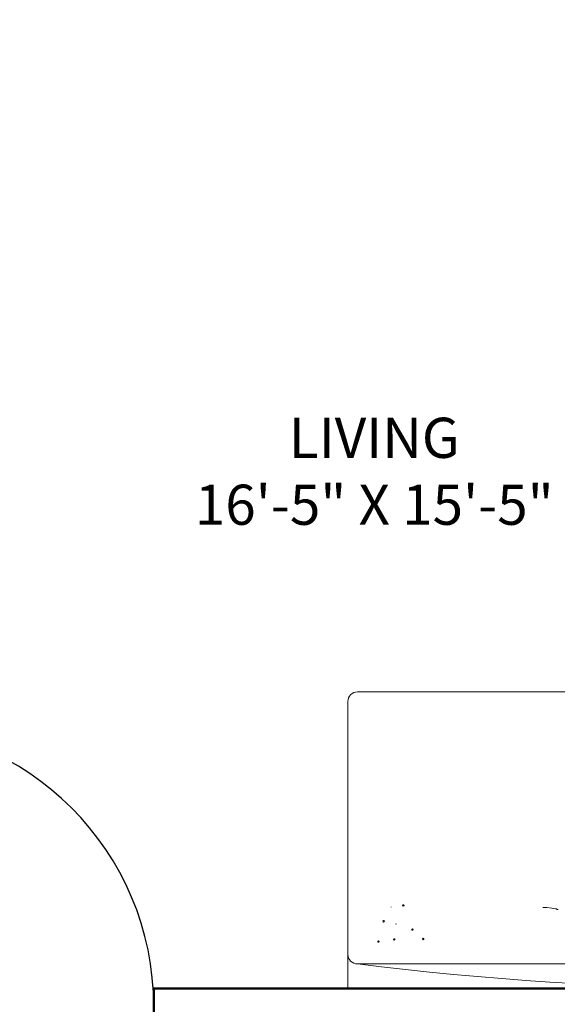
# Model space of a CAD drawing. Units: inches. Extents: x -466983 to 1020, y 324 to 318697.
# Tile 19 of 97: x 641 to 721, y 511 to 658. Entities that reach past the tile are written whole.
import ezdxf

# ---------------------------------------------------------------- set-up
doc = ezdxf.new("R2010")
doc.units = ezdxf.units.IN
doc.header["$MEASUREMENT"] = 0
for name, color, linetype, lineweight in [('A-ANNO-DIMS', 2, 'Continuous', 18), ('A-AREA-IDEN', 7, 'Continuous', 25), ('A-DOOR', 3, 'Continuous', 25), ('A-FLOR-PATT', 252, 'Continuous', 13), ('A-FURN', 8, 'Continuous', 18), ('A-WALL', 7, 'Continuous', 50)]:
    doc.layers.add(name, color=color, linetype=linetype, lineweight=lineweight)
doc.styles.get("Standard").update_dxf_attribs({"font": 'arial.ttf'})
doc.dimstyles.get("Standard").update_dxf_attribs({"dimtxt": 6, "dimasz": 4, "dimexe": 3, "dimexo": 3, "dimgap": 0.09, "dimtad": 0, "dimtih": 1, "dimtoh": 1, "dimdec": 1, "dimzin": 0, "dimdsep": 46, "dimlunit": 3, "dimtxsty": 'Standard', "dimcen": 0.09, "dimadec": 0, "dimazin": 0, "dimtfac": 1, "dimtdec": 1, "dimtofl": 0, "dimtmove": 0, "dimatfit": 3, "dimfxl": 1, "dimtolj": 1, "dimtzin": 0, "dimarcsym": 0})

# ---------------------------------------------------------------- blocks, each defined once
blk = doc.blocks.new('L Shaped Sofa')
at = {"ltscale": 2}
for p, q in [((2356.7, 767.57), (2377.23, 767.57)), ((2377.23, 767.57), (2392.32, 767.57)), ((2355.26, 760.48), (2355.26, 766.13)), ((2355.26, 760.48), (2355.26, 736.26)), ((2355.26, 728.35), (2355.26, 736.26)), ((2384.4, 735.35), (2384.99, 735.35)), ((2384.99, 735.35), (2385.77, 735.24)), ((2385.77, 735.24), (2386.06, 735.18)), ((2386.06, 735.18), (2386.3, 735.13)), ((2386.3, 735.13), (2386.45, 735.13)), ((2386.45, 735.13), (2386.55, 735.07)), ((2386.55, 735.07), (2386.69, 735.07)), ((2355.26, 723.23), (2355.26, 728.35)), ((2356.7, 726.92), (2377.23, 726.92)), ((2393.28, 726.92), (2377.23, 726.92)), ((2355.26, 723.23), (2377.23, 723.23)), ((2475.26, 723.23), (2377.23, 723.23))]:
    blk.add_line(p, q, dxfattribs=at)
for centre, radius, start, end in [((2356.7, 766.13), 1.43, 90, 180), ((2363.56, 735.66), 0.106, 90, 270), ((2363.56, 735.66), 0.106, 270, 90), ((2361.75, 735.43), 0.0177, 90, 270), ((2361.75, 735.43), 0.0177, 270, 90), ((2360.62, 733.28), 0.106, 90, 270), ((2360.62, 733.28), 0.106, 270, 90), ((2362.45, 732.89), 0.0177, 90, 270), ((2362.45, 732.89), 0.0177, 270, 90), ((2364.92, 732.04), 0.106, 90, 270), ((2364.92, 732.04), 0.106, 270, 90), ((2359.84, 730.26), 0.106, 90, 270), ((2359.84, 730.26), 0.106, 270, 90), ((2362.21, 730.57), 0.106, 90, 270), ((2362.21, 730.57), 0.106, 270, 90), ((2366.53, 730.64), 0.106, 90, 270), ((2366.53, 730.64), 0.106, 270, 90), ((2356.7, 728.35), 1.43, 180, 270), ((2416.36, 1205.03), 481.82, 262.8867, 276.632)]:
    blk.add_arc(centre, radius, start, end, dxfattribs=at)
blk = doc.blocks.new('*U41')
for p, q in [((0, 0), (0, -6)), ((40, 0), (40, -6))]:
    blk.add_line(p, q)
blk.add_lwpolyline([(0, 0), (0, 40), (1.75, 40), (1.75, 0)], close=True)
blk.add_arc((0, 0), 40, 0, 90)
blk = doc.blocks.new('*D70')
at = {"layer": 'A-ANNO-DIMS', "color": 0, "lineweight": -2, "transparency": 16777216}
for p, q in [((689.81, 508.69), (689.81, 490)), ((810.97, 508.69), (810.97, 490)), ((693.81, 493), (744.53, 493)), ((806.97, 493), (756.24, 493))]:
    blk.add_line(p, q, dxfattribs=at)
at = {"layer": 'A-ANNO-DIMS', "color": 0, "transparency": 16777216}
for points in [[(693.81, 493.67), (693.81, 492.34), (689.81, 493)], [(806.97, 493.67), (806.97, 492.34), (810.97, 493)]]:
    blk.add_solid(points, dxfattribs=at)
at = {"layer": 'Defpoints', "color": 0, "transparency": 16777216}
for p in [(689.81, 511.69), (810.97, 511.69), (810.97, 493)]:
    blk.add_point(p, dxfattribs=at)
at = {"layer": 'A-ANNO-DIMS', "color": 0, "transparency": 16777216, "insert": (750.39, 493), "char_height": 6, "attachment_point": 5}
blk.add_mtext('\\A1;121', dxfattribs=at)

msp = doc.modelspace()

# ---------------------------------------------------------------- hatches: boundary and pattern name
at = {"layer": 'A-FLOR-PATT', "transparency": 33554572}
h = msp.add_hatch(dxfattribs=at)
h.set_pattern_fill('ANSI37', color=256, scale=30)
h.set_pattern_definition([(45, (-1212.4137, -290.035), (-2.6516504, 2.6516504), []), (135, (-1212.4137, -290.035), (-2.6516504, -2.6516504), [])])
h.paths.add_polyline_path([(901.81, 1075.94), (900.61, 1075.94), (900.61, 1065.39), (899.39, 1065.39), (898.09, 1065.39), (892.84, 1058.71, -0.258377), (892.19, 1058.35), (879.98, 1058.35, -0.20177), (879.44, 1058.58), (874.08, 1065.39), (872.78, 1065.39), (871.56, 1065.39), (871.56, 1075.94), (813.81, 1075.94), (813.81, 1044.79), (832.39, 1044.79, -0.394795), (848.66, 1028.54), (848.66, 1009.94), (901.81, 1009.94), (901.81, 1015.94), (901.31, 1015.94), (871.31, 1015.94), (871.31, 1017.25), (871.33, 1017.25, -0.401453), (901.31, 1045.94), (901.81, 1045.94)])
edge = h.paths.add_edge_path(flags=16)
edge.add_line((847.77, 1068.95), (847.77, 1073.71))
edge.add_arc((849.23, 1073.71), 1.45, 90, 180, ccw=False)
edge.add_line((849.23, 1075.16), (864.49, 1075.16))
edge.add_arc((864.49, 1073.71), 1.45, 0, 90, ccw=False)
edge.add_line((865.95, 1073.71), (865.95, 1069))
edge.add_arc((832.64, 1068.98), 33.3, -20.6123, 0.0472, ccw=False)
edge.add_ellipse((856.86, 1058.48), major_axis=(0, 10.21), ratio=0.685919, start_angle=100.0088, end_angle=259.9912, ccw=False)
edge.add_arc((881.07, 1068.98), 33.3, 180.0472, 200.6123, ccw=False)
h.paths.add_polyline_path([(853.15, 1066.48), (853.15, 1066.45), (853.15, 1066.45, 0.433107), (852.92, 1066.68), (852.92, 1066.45), (853.15, 1066.45), (853.15, 1066.48), (853.09, 1066.61, 0.697939), (852.7, 1066.45), (852.7, 1066.45), (852.7, 1066.48), (852.92, 1067), (852.92, 1066.68, -0.396254)], flags=0)
h.paths.add_polyline_path([(861.02, 1066.48), (861.02, 1066.45), (861.02, 1066.45, 0.416404), (860.8, 1066.68), (860.8, 1066.45), (861.02, 1066.45), (861.02, 1066.48), (860.97, 1066.61, 0.713344), (860.57, 1066.45), (860.57, 1066.45), (860.57, 1066.48), (860.8, 1067), (860.8, 1066.68, -0.379973)], flags=0)
edge = h.paths.add_edge_path(flags=0)
edge.add_spline(control_points=[(861.13, 1065.79), (861.47, 1065.25), (861.61, 1065.02), (861.98, 1064.37), (862.19, 1063.94), (862.56, 1063.04), (862.72, 1062.56), (862.99, 1061.58), (863.09, 1061.07), (863.25, 1060.03), (863.29, 1059.5), (863.33, 1058.44), (863.32, 1057.91), (863.24, 1056.85), (863.17, 1056.33), (862.97, 1055.31), (862.84, 1054.81), (862.54, 1053.85), (862.36, 1053.39), (861.95, 1052.52), (861.73, 1052.12), (861.23, 1051.36), (860.97, 1051.02), (860.4, 1050.39), (860.11, 1050.12), (859.49, 1049.65), (859.18, 1049.45), (858.53, 1049.13), (858.2, 1049.01), (857.53, 1048.85), (857.2, 1048.81), (856.52, 1048.81), (856.19, 1048.85), (855.52, 1049.01), (855.19, 1049.13), (854.54, 1049.45), (854.23, 1049.64), (853.61, 1050.12), (853.32, 1050.39), (852.75, 1051.01), (852.49, 1051.36), (852, 1052.11), (851.77, 1052.52), (851.36, 1053.39), (851.18, 1053.85), (850.88, 1054.81), (850.75, 1055.31), (850.55, 1056.33), (850.48, 1056.85), (850.4, 1057.9), (850.39, 1058.44), (850.43, 1059.5), (850.47, 1060.03), (850.63, 1061.07), (850.73, 1061.58), (851, 1062.56), (851.16, 1063.04), (851.53, 1063.94), (851.73, 1064.37), (852.11, 1065.02), (852.25, 1065.25), (852.61, 1065.73)], knot_values=[3.915332, 3.915332, 3.915332, 3.915332, 4.013468, 4.013468, 4.175532, 4.175532, 4.337596, 4.337596, 4.49966, 4.49966, 4.661724, 4.661724, 4.823788, 4.823788, 4.985852, 4.985852, 5.147916, 5.147916, 5.30998, 5.30998, 5.472044, 5.472044, 5.634109, 5.634109, 5.796173, 5.796173, 5.958237, 5.958237, 6.120301, 6.120301, 6.282365, 6.282365, 6.444429, 6.444429, 6.606493, 6.606493, 6.768557, 6.768557, 6.930621, 6.930621, 7.092685, 7.092685, 7.254749, 7.254749, 7.416813, 7.416813, 7.578878, 7.578878, 7.740942, 7.740942, 7.903006, 7.903006, 8.06507, 8.06507, 8.227134, 8.227134, 8.389198, 8.389198, 8.551262, 8.551262, 8.65037, 8.65037, 8.65037, 8.65037], degree=3, periodic=0)
edge.add_line((852.64, 1065.79), (861.13, 1065.79))
edge = h.paths.add_edge_path(flags=0)
edge.add_ellipse((856.85, 1057.74), major_axis=(0, 7.79), ratio=0.687861, start_angle=0, end_angle=360)
h.paths.add_polyline_path([(848.86, 1069.39), (848.86, 1073.96, -0.414214), (849.95, 1075.05), (863.77, 1075.05, -0.414214), (864.86, 1073.96), (864.86, 1069.39, -0.388936), (864.52, 1069.03, -0.043561), (849.2, 1069.03, -0.388936)], flags=0)
h.paths.add_polyline_path([(853.1, 1068.11, -1), (852.68, 1068.11, -1)], flags=0)
edge = h.paths.add_edge_path(flags=0)
edge.add_ellipse((856.86, 1057.34), major_axis=(0, 2.21), ratio=0.657164, start_angle=0, end_angle=360)
h.paths.add_polyline_path([(861.04, 1068.11, -1), (860.62, 1068.11, -1)], flags=0)
edge = h.paths.add_edge_path()
edge.add_line((573.95, 1057.34), (573.95, 1075.94))
edge.add_line((573.95, 1075.94), (558.73, 1075.94))
edge.add_line((558.73, 1075.94), (558.73, 1065.39))
edge.add_line((558.73, 1065.39), (557.51, 1065.39))
edge.add_line((557.51, 1065.39), (556.21, 1065.39))
edge.add_line((556.21, 1065.39), (550.95, 1058.71))
edge.add_arc((550.3, 1059.12), 0.765, 270, 327.9483, ccw=False)
edge.add_line((550.3, 1058.35), (538.1, 1058.35))
edge.add_arc((538.1, 1059.12), 0.765, 224.3704, 270, ccw=False)
edge.add_line((537.55, 1058.58), (532.2, 1065.39))
edge.add_line((532.2, 1065.39), (530.9, 1065.39))
edge.add_line((530.9, 1065.39), (529.67, 1065.39))
edge.add_line((529.67, 1065.39), (529.67, 1075.94))
edge.add_line((529.67, 1075.94), (520.81, 1075.94))
edge.add_line((520.81, 1075.94), (520.81, 1045.94))
edge.add_line((520.81, 1045.94), (521.31, 1045.94))
edge.add_arc((521.31, 1015.94), 30, 2.5075, 90, ccw=False)
edge.add_line((551.28, 1017.25), (551.31, 1017.25))
edge.add_line((551.31, 1017.25), (551.31, 1015.94))
edge.add_line((551.31, 1015.94), (520.81, 1015.94))
edge.add_line((520.81, 1015.94), (520.81, 1009.94))
edge.add_line((520.81, 1009.94), (559.19, 1010.4))
edge.add_arc((559.19, 1011.86), 1.45, 180, 270, ccw=False)
edge.add_line((557.74, 1011.86), (557.74, 1016.56))
edge.add_arc((591.04, 1016.59), 33.3, 159.3877, 180.0472, ccw=False)
edge.add_ellipse((566.82, 1027.08), major_axis=(0, 10.21), ratio=0.685919, start_angle=280.0088, end_angle=439.9912, ccw=False)
edge.add_arc((542.61, 1016.59), 33.3, 0.0472, 20.6123, ccw=False)
edge.add_line((575.91, 1016.62), (575.91, 1011.86))
edge.add_arc((574.46, 1011.86), 1.45, -90, 0, ccw=False)
edge.add_line((574.46, 1010.4), (608.81, 1009.94))
edge.add_line((608.81, 1009.94), (608.81, 1041.09))
edge.add_line((608.81, 1041.09), (590.22, 1041.09))
edge.add_arc((590.78, 1057.91), 16.83, 181.9277, 268.1032, ccw=False)
edge = h.paths.add_edge_path()
edge.add_ellipse((494.24, 583.62), major_axis=(0, 10.21), ratio=0.685919, start_angle=280.0088, end_angle=439.9912, ccw=False)
edge.add_arc((470.03, 573.12), 33.3, 0.0472, 20.6123, ccw=False)
edge.add_line((503.33, 573.15), (503.33, 568.39))
edge.add_arc((501.88, 568.39), 1.45, -90, 0, ccw=False)
edge.add_line((501.88, 566.94), (539.81, 566.94))
edge.add_line((539.81, 566.94), (539.81, 572.94))
edge.add_line((539.81, 572.94), (539.31, 572.94))
edge.add_line((539.31, 572.94), (509.31, 572.94))
edge.add_line((509.31, 572.94), (509.31, 574.25))
edge.add_line((509.31, 574.25), (509.33, 574.25))
edge.add_arc((539.31, 572.94), 30, 90, 177.4925, ccw=False)
edge.add_line((539.31, 602.94), (539.81, 602.94))
edge.add_line((539.81, 602.94), (539.81, 626.94))
edge.add_line((539.81, 626.94), (531.77, 626.94))
edge.add_line((531.77, 626.94), (531.77, 616.39))
edge.add_line((531.77, 616.39), (530.55, 616.39))
edge.add_line((530.55, 616.39), (529.25, 616.39))
edge.add_line((529.25, 616.39), (523.71, 609.35))
edge.add_line((523.71, 609.35), (510.78, 609.35))
edge.add_line((510.78, 609.35), (505.24, 616.39))
edge.add_line((505.24, 616.39), (503.94, 616.39))
edge.add_line((503.94, 616.39), (502.72, 616.39))
edge.add_line((502.72, 616.39), (502.72, 626.94))
edge.add_line((502.72, 626.94), (481.7, 626.94))
edge.add_line((481.7, 626.94), (481.7, 611))
edge.add_arc((467.27, 611.47), 14.44, 271.9277, 358.1032, ccw=False)
edge.add_line((467.76, 597.05), (451.81, 597.05))
edge.add_line((451.81, 597.05), (451.81, 584.4))
edge.add_line((451.81, 584.4), (451.81, 566.94))
edge.add_line((451.81, 566.94), (486.61, 566.94))
edge.add_arc((486.61, 568.39), 1.45, 180, 270, ccw=False)
edge.add_line((485.16, 568.39), (485.16, 573.1))
edge.add_arc((518.46, 573.12), 33.3, 159.3877, 180.0472, ccw=False)
h.paths.add_polyline_path([(836.26, 1020.73), (879.89, 1020.73), (879.89, 1039.39), (836.26, 1039.39)], flags=25)
h.paths.add_polyline_path([(549.99, 1036.75), (593.61, 1036.75), (593.61, 1055.41), (549.99, 1055.41)], flags=24)
h.paths.add_polyline_path([(475.12, 595.6), (518.75, 595.6), (518.75, 614.25), (475.12, 614.25)], flags=24)

# ---------------------------------------------------------------- linework, layer by layer
at = {"layer": 'A-WALL'}
for p in [(809.81, 512.94), (660.81, 503.94)]:
    msp.add_line(p, (660.81, 512.94), dxfattribs=at)

# ---------------------------------------------------------------- block references
at = {"layer": 'A-DOOR', "xscale": 1.05, "yscale": 1.05, "zscale": 1.05}
msp.add_blockref('*U41', (618.81, 510.24), dxfattribs=at)
at = {"layer": 'A-FURN'}
msp.add_blockref('L Shaped Sofa', (-1665.46, -210.29), dxfattribs=at)

# ---------------------------------------------------------------- texts
at = {"layer": 'A-AREA-IDEN', "insert": (578.98, 598.24), "char_height": 6, "attachment_point": 1}
msp.add_mtext_dynamic_manual_height_columns('\\pxqc;{\\fArial|b1|i0|c0|p34;LIVING\\P16\'-5" X 15\'-5"}', width=229.5583, gutter_width=1, heights=[0], dxfattribs=at)

# ---------------------------------------------------------------- dimensions: what is measured, and where the dimension line sits
at = {"layer": 'A-ANNO-DIMS'}
dim = msp.add_linear_dim(base=(810.97, 493), p1=(689.81, 511.69), p2=(810.97, 511.69), dimstyle='Standard', override={"dimdec": 0, "dimlfac": 1, "dimrnd": 0, "dimzin": 0, "dimdsep": 46, "dimlunit": 2}, dxfattribs=at)
dim.commit()
dim.dimension.update_dxf_attribs({"geometry": '*D70', "text_midpoint": (750.39, 493)})

doc.saveas('drawing.dxf')
